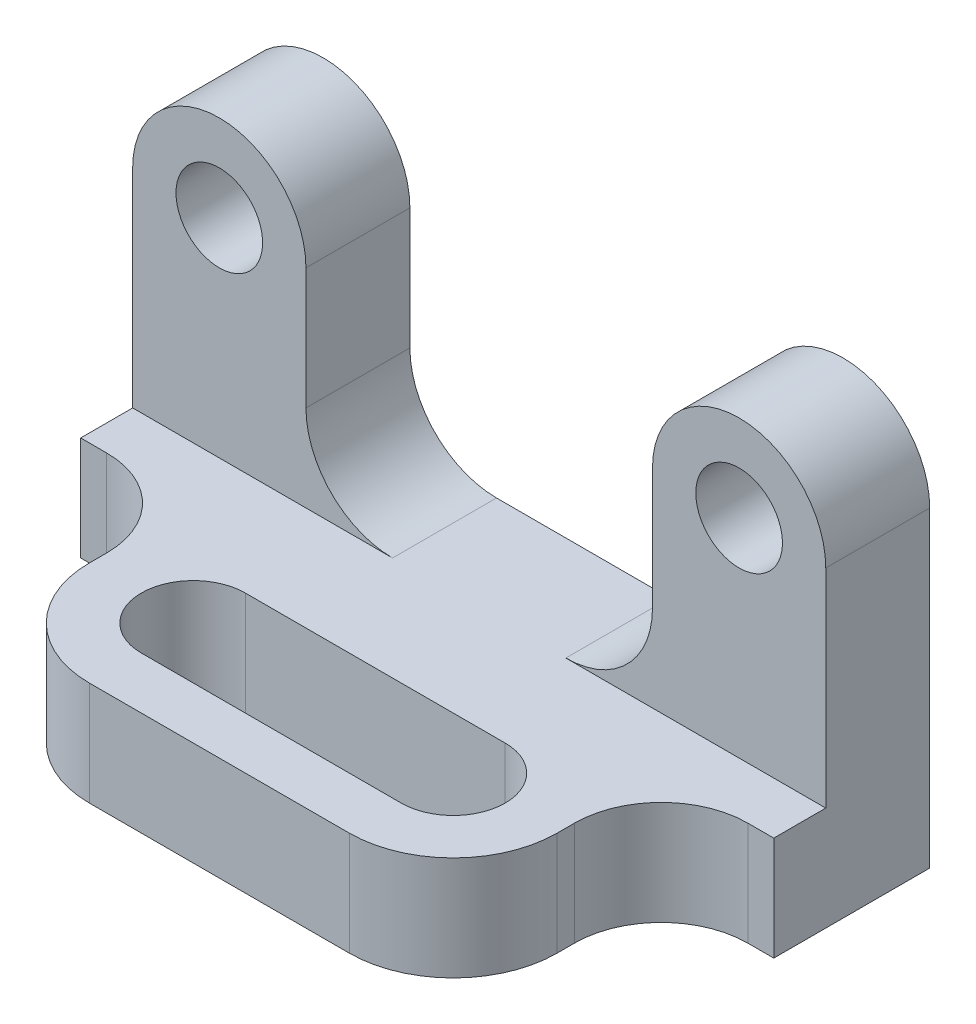
ISO-10303-21;
HEADER;
FILE_DESCRIPTION(('STEP AP214'),'2;1');
FILE_NAME('part.step','',(''),(''),'','','');
FILE_SCHEMA(('AUTOMOTIVE_DESIGN { 1 0 10303 214 1 1 1 1 }'));
ENDSEC;
DATA;
#1=APPLICATION_CONTEXT('core data for automotive mechanical design processes');
#2=APPLICATION_PROTOCOL_DEFINITION('international standard','automotive_design',2000,#1);
#3=PRODUCT_CONTEXT('',#1,'mechanical');
#4=PRODUCT('Part','Part','',(#3));
#5=PRODUCT_RELATED_PRODUCT_CATEGORY('part','',(#4));
#6=PRODUCT_DEFINITION_FORMATION('','',#4);
#7=PRODUCT_DEFINITION_CONTEXT('part definition',#1,'design');
#8=PRODUCT_DEFINITION('design','',#6,#7);
#9=PRODUCT_DEFINITION_SHAPE('','',#8);
#10=(LENGTH_UNIT() NAMED_UNIT(*) SI_UNIT(.MILLI.,.METRE.));
#11=(NAMED_UNIT(*) PLANE_ANGLE_UNIT() SI_UNIT($,.RADIAN.));
#12=(NAMED_UNIT(*) SI_UNIT($,.STERADIAN.) SOLID_ANGLE_UNIT());
#13=UNCERTAINTY_MEASURE_WITH_UNIT(LENGTH_MEASURE(1.E-05),#10,'distance_accuracy_value','');
#14=(GEOMETRIC_REPRESENTATION_CONTEXT(3) GLOBAL_UNCERTAINTY_ASSIGNED_CONTEXT((#13)) GLOBAL_UNIT_ASSIGNED_CONTEXT((#10,
#11,#12)) REPRESENTATION_CONTEXT('',''));
#15=CARTESIAN_POINT('',(0.,0.,0.));
#16=DIRECTION('',(0.,0.,1.));
#17=DIRECTION('',(1.,0.,0.));
#18=AXIS2_PLACEMENT_3D('',#15,#16,#17);
#19=CARTESIAN_POINT('',(0.,3.,0.));
#20=DIRECTION('',(0.,1.,0.));
#21=DIRECTION('',(0.,0.,1.));
#22=AXIS2_PLACEMENT_3D('',#19,#20,#21);
#23=PLANE('',#22);
#24=CARTESIAN_POINT('',(7.5,3.,12.));
#25=DIRECTION('',(0.,1.,0.));
#26=DIRECTION('',(0.,0.,1.));
#27=AXIS2_PLACEMENT_3D('',#24,#25,#26);
#28=CIRCLE('',#27,3.);
#29=CARTESIAN_POINT('',(7.5,3.,15.));
#30=VERTEX_POINT('',#29);
#31=CARTESIAN_POINT('',(7.5,3.,8.99999999999999));
#32=VERTEX_POINT('',#31);
#33=EDGE_CURVE('E176',#30,#32,#28,.T.);
#34=ORIENTED_EDGE('',*,*,#33,.F.);
#35=DIRECTION('',(1.,0.,0.));
#36=VECTOR('',#35,1.);
#37=CARTESIAN_POINT('',(0.,3.,15.));
#38=LINE('',#37,#36);
#39=CARTESIAN_POINT('',(-7.5,3.,15.));
#40=VERTEX_POINT('',#39);
#41=EDGE_CURVE('E164',#40,#30,#38,.T.);
#42=ORIENTED_EDGE('',*,*,#41,.F.);
#43=CARTESIAN_POINT('',(-7.5,3.,12.));
#44=DIRECTION('',(0.,1.,0.));
#45=DIRECTION('',(0.,0.,1.));
#46=AXIS2_PLACEMENT_3D('',#43,#44,#45);
#47=CIRCLE('',#46,3.);
#48=CARTESIAN_POINT('',(-7.5,3.,8.99999999999999));
#49=VERTEX_POINT('',#48);
#50=EDGE_CURVE('E179',#49,#40,#47,.T.);
#51=ORIENTED_EDGE('',*,*,#50,.F.);
#52=DIRECTION('',(1.,0.,0.));
#53=VECTOR('',#52,1.);
#54=CARTESIAN_POINT('',(0.,3.,8.99999999999999));
#55=LINE('',#54,#53);
#56=EDGE_CURVE('E64',#49,#32,#55,.T.);
#57=ORIENTED_EDGE('',*,*,#56,.T.);
#58=EDGE_LOOP('',(#34,#42,#51,#57));
#59=FACE_BOUND('',#58,.T.);
#60=DIRECTION('',(0.,0.,-1.));
#61=VECTOR('',#60,1.);
#62=CARTESIAN_POINT('',(20.,3.,0.));
#63=LINE('',#62,#61);
#64=CARTESIAN_POINT('',(20.,3.,5.99999999999999));
#65=VERTEX_POINT('',#64);
#66=CARTESIAN_POINT('',(20.,3.,3.));
#67=VERTEX_POINT('',#66);
#68=EDGE_CURVE('E354',#65,#67,#63,.T.);
#69=ORIENTED_EDGE('',*,*,#68,.T.);
#70=DIRECTION('',(-1.,0.,0.));
#71=VECTOR('',#70,1.);
#72=CARTESIAN_POINT('',(0.,3.,3.));
#73=LINE('',#72,#71);
#74=CARTESIAN_POINT('',(4.99999999999997,3.,3.));
#75=VERTEX_POINT('',#74);
#76=EDGE_CURVE('E188',#67,#75,#73,.T.);
#77=ORIENTED_EDGE('',*,*,#76,.T.);
#78=DIRECTION('',(0.,0.,1.));
#79=VECTOR('',#78,1.);
#80=CARTESIAN_POINT('',(5.,3.,-3.));
#81=LINE('',#80,#79);
#82=CARTESIAN_POINT('',(4.99999999999997,3.,-3.));
#83=VERTEX_POINT('',#82);
#84=EDGE_CURVE('E47',#75,#83,#81,.F.);
#85=ORIENTED_EDGE('',*,*,#84,.T.);
#86=DIRECTION('',(1.,0.,0.));
#87=VECTOR('',#86,1.);
#88=CARTESIAN_POINT('',(0.,3.,-3.));
#89=LINE('',#88,#87);
#90=CARTESIAN_POINT('',(-4.99999999999997,3.,-3.));
#91=VERTEX_POINT('',#90);
#92=EDGE_CURVE('E260',#91,#83,#89,.T.);
#93=ORIENTED_EDGE('',*,*,#92,.F.);
#94=DIRECTION('',(0.,0.,1.));
#95=VECTOR('',#94,1.);
#96=CARTESIAN_POINT('',(-5.,3.,-3.));
#97=LINE('',#96,#95);
#98=CARTESIAN_POINT('',(-4.99999999999997,3.,3.));
#99=VERTEX_POINT('',#98);
#100=EDGE_CURVE('E11',#99,#91,#97,.F.);
#101=ORIENTED_EDGE('',*,*,#100,.F.);
#102=CARTESIAN_POINT('',(-20.,3.,3.));
#103=VERTEX_POINT('',#102);
#104=EDGE_CURVE('E344',#99,#103,#73,.T.);
#105=ORIENTED_EDGE('',*,*,#104,.T.);
#106=DIRECTION('',(0.,0.,1.));
#107=VECTOR('',#106,1.);
#108=CARTESIAN_POINT('',(-20.,3.,0.));
#109=LINE('',#108,#107);
#110=CARTESIAN_POINT('',(-20.,3.,6.));
#111=VERTEX_POINT('',#110);
#112=EDGE_CURVE('E356',#103,#111,#109,.T.);
#113=ORIENTED_EDGE('',*,*,#112,.T.);
#114=DIRECTION('',(1.,0.,0.));
#115=VECTOR('',#114,1.);
#116=CARTESIAN_POINT('',(0.,3.,6.));
#117=LINE('',#116,#115);
#118=CARTESIAN_POINT('',(-18.5,3.,6.));
#119=VERTEX_POINT('',#118);
#120=EDGE_CURVE('E358',#111,#119,#117,.T.);
#121=ORIENTED_EDGE('',*,*,#120,.T.);
#122=CARTESIAN_POINT('',(-18.5,3.,11.));
#123=DIRECTION('',(0.,1.,0.));
#124=DIRECTION('',(0.,0.,1.));
#125=AXIS2_PLACEMENT_3D('',#122,#123,#124);
#126=CIRCLE('',#125,5.);
#127=CARTESIAN_POINT('',(-13.5,3.,11.));
#128=VERTEX_POINT('',#127);
#129=EDGE_CURVE('E363',#128,#119,#126,.T.);
#130=ORIENTED_EDGE('',*,*,#129,.F.);
#131=DIRECTION('',(0.,0.,-1.));
#132=VECTOR('',#131,1.);
#133=CARTESIAN_POINT('',(-13.5,3.,0.));
#134=LINE('',#133,#132);
#135=CARTESIAN_POINT('',(-13.5,3.,12.));
#136=VERTEX_POINT('',#135);
#137=EDGE_CURVE('E365',#136,#128,#134,.T.);
#138=ORIENTED_EDGE('',*,*,#137,.F.);
#139=CARTESIAN_POINT('',(-7.5,3.,12.));
#140=DIRECTION('',(0.,1.,0.));
#141=DIRECTION('',(0.,0.,1.));
#142=AXIS2_PLACEMENT_3D('',#139,#140,#141);
#143=CIRCLE('',#142,6.);
#144=CARTESIAN_POINT('',(-7.49999999999996,3.,18.));
#145=VERTEX_POINT('',#144);
#146=EDGE_CURVE('E224',#145,#136,#143,.F.);
#147=ORIENTED_EDGE('',*,*,#146,.F.);
#148=DIRECTION('',(1.,0.,0.));
#149=VECTOR('',#148,1.);
#150=CARTESIAN_POINT('',(0.,3.,18.));
#151=LINE('',#150,#149);
#152=CARTESIAN_POINT('',(7.49999999999996,3.,18.));
#153=VERTEX_POINT('',#152);
#154=EDGE_CURVE('E343',#145,#153,#151,.T.);
#155=ORIENTED_EDGE('',*,*,#154,.T.);
#156=CARTESIAN_POINT('',(7.5,3.,12.));
#157=DIRECTION('',(0.,1.,0.));
#158=DIRECTION('',(0.,0.,1.));
#159=AXIS2_PLACEMENT_3D('',#156,#157,#158);
#160=CIRCLE('',#159,6.);
#161=CARTESIAN_POINT('',(13.5,3.,12.));
#162=VERTEX_POINT('',#161);
#163=EDGE_CURVE('E347',#162,#153,#160,.F.);
#164=ORIENTED_EDGE('',*,*,#163,.F.);
#165=DIRECTION('',(0.,0.,-1.));
#166=VECTOR('',#165,1.);
#167=CARTESIAN_POINT('',(13.5,3.,0.));
#168=LINE('',#167,#166);
#169=CARTESIAN_POINT('',(13.5,3.,11.));
#170=VERTEX_POINT('',#169);
#171=EDGE_CURVE('E349',#162,#170,#168,.T.);
#172=ORIENTED_EDGE('',*,*,#171,.T.);
#173=CARTESIAN_POINT('',(18.5,3.,11.));
#174=DIRECTION('',(0.,1.,0.));
#175=DIRECTION('',(0.,0.,1.));
#176=AXIS2_PLACEMENT_3D('',#173,#174,#175);
#177=CIRCLE('',#176,5.);
#178=CARTESIAN_POINT('',(18.5,3.,5.99999999999999));
#179=VERTEX_POINT('',#178);
#180=EDGE_CURVE('E351',#170,#179,#177,.F.);
#181=ORIENTED_EDGE('',*,*,#180,.T.);
#182=DIRECTION('',(1.,0.,0.));
#183=VECTOR('',#182,1.);
#184=CARTESIAN_POINT('',(0.,3.,5.99999999999999));
#185=LINE('',#184,#183);
#186=EDGE_CURVE('E352',#179,#65,#185,.T.);
#187=ORIENTED_EDGE('',*,*,#186,.T.);
#188=EDGE_LOOP('',(#69,#77,#85,#93,#101,#105,#113,#121,#130,#138,#147,#155,#164,#172,#181,#187));
#189=FACE_BOUND('',#188,.T.);
#190=ADVANCED_FACE('F41',(#59,#189),#23,.T.);
#191=CARTESIAN_POINT('',(7.5,3.,12.));
#192=DIRECTION('',(0.,-1.,0.));
#193=DIRECTION('',(0.,0.,-1.));
#194=AXIS2_PLACEMENT_3D('',#191,#192,#193);
#195=CYLINDRICAL_SURFACE('',#194,3.);
#196=CARTESIAN_POINT('',(7.5,-3.,12.));
#197=DIRECTION('',(0.,1.,0.));
#198=DIRECTION('',(0.,0.,1.));
#199=AXIS2_PLACEMENT_3D('',#196,#197,#198);
#200=CIRCLE('',#199,3.);
#201=CARTESIAN_POINT('',(7.5,-3.,15.));
#202=VERTEX_POINT('',#201);
#203=CARTESIAN_POINT('',(7.5,-3.,8.99999999999999));
#204=VERTEX_POINT('',#203);
#205=EDGE_CURVE('E214',#202,#204,#200,.T.);
#206=ORIENTED_EDGE('',*,*,#205,.F.);
#207=DIRECTION('',(0.,-1.,0.));
#208=VECTOR('',#207,1.);
#209=CARTESIAN_POINT('',(7.5,3.,15.));
#210=LINE('',#209,#208);
#211=EDGE_CURVE('E175',#30,#202,#210,.T.);
#212=ORIENTED_EDGE('',*,*,#211,.F.);
#213=ORIENTED_EDGE('',*,*,#33,.T.);
#214=DIRECTION('',(0.,-1.,0.));
#215=VECTOR('',#214,1.);
#216=CARTESIAN_POINT('',(7.5,3.,8.99999999999999));
#217=LINE('',#216,#215);
#218=EDGE_CURVE('E120',#32,#204,#217,.T.);
#219=ORIENTED_EDGE('',*,*,#218,.T.);
#220=EDGE_LOOP('',(#206,#212,#213,#219));
#221=FACE_BOUND('',#220,.T.);
#222=ADVANCED_FACE('F368',(#221),#195,.F.);
#223=CARTESIAN_POINT('',(0.,3.,15.));
#224=DIRECTION('',(0.,0.,-1.));
#225=DIRECTION('',(-1.,0.,0.));
#226=AXIS2_PLACEMENT_3D('',#223,#224,#225);
#227=PLANE('',#226);
#228=DIRECTION('',(1.,0.,0.));
#229=VECTOR('',#228,1.);
#230=CARTESIAN_POINT('',(0.,-3.,15.));
#231=LINE('',#230,#229);
#232=CARTESIAN_POINT('',(-7.5,-3.,15.));
#233=VERTEX_POINT('',#232);
#234=EDGE_CURVE('E170',#233,#202,#231,.T.);
#235=ORIENTED_EDGE('',*,*,#234,.F.);
#236=DIRECTION('',(0.,-1.,0.));
#237=VECTOR('',#236,1.);
#238=CARTESIAN_POINT('',(-7.5,3.,15.));
#239=LINE('',#238,#237);
#240=EDGE_CURVE('E165',#40,#233,#239,.T.);
#241=ORIENTED_EDGE('',*,*,#240,.F.);
#242=ORIENTED_EDGE('',*,*,#41,.T.);
#243=ORIENTED_EDGE('',*,*,#211,.T.);
#244=EDGE_LOOP('',(#235,#241,#242,#243));
#245=FACE_BOUND('',#244,.T.);
#246=ADVANCED_FACE('F163',(#245),#227,.T.);
#247=CARTESIAN_POINT('',(-7.5,3.,12.));
#248=DIRECTION('',(0.,-1.,0.));
#249=DIRECTION('',(0.,0.,-1.));
#250=AXIS2_PLACEMENT_3D('',#247,#248,#249);
#251=CYLINDRICAL_SURFACE('',#250,3.);
#252=CARTESIAN_POINT('',(-7.5,-3.,12.));
#253=DIRECTION('',(0.,1.,0.));
#254=DIRECTION('',(0.,0.,1.));
#255=AXIS2_PLACEMENT_3D('',#252,#253,#254);
#256=CIRCLE('',#255,3.);
#257=CARTESIAN_POINT('',(-7.5,-3.,8.99999999999999));
#258=VERTEX_POINT('',#257);
#259=EDGE_CURVE('E218',#258,#233,#256,.T.);
#260=ORIENTED_EDGE('',*,*,#259,.F.);
#261=DIRECTION('',(0.,-1.,0.));
#262=VECTOR('',#261,1.);
#263=CARTESIAN_POINT('',(-7.5,3.,8.99999999999999));
#264=LINE('',#263,#262);
#265=EDGE_CURVE('E172',#49,#258,#264,.T.);
#266=ORIENTED_EDGE('',*,*,#265,.F.);
#267=ORIENTED_EDGE('',*,*,#50,.T.);
#268=ORIENTED_EDGE('',*,*,#240,.T.);
#269=EDGE_LOOP('',(#260,#266,#267,#268));
#270=FACE_BOUND('',#269,.T.);
#271=ADVANCED_FACE('F178',(#270),#251,.F.);
#272=CARTESIAN_POINT('',(-7.5,3.,12.));
#273=DIRECTION('',(0.,-1.,0.));
#274=DIRECTION('',(0.,0.,-1.));
#275=AXIS2_PLACEMENT_3D('',#272,#273,#274);
#276=CYLINDRICAL_SURFACE('',#275,6.);
#277=CARTESIAN_POINT('',(-7.5,-3.,12.));
#278=DIRECTION('',(0.,1.,0.));
#279=DIRECTION('',(0.,0.,1.));
#280=AXIS2_PLACEMENT_3D('',#277,#278,#279);
#281=CIRCLE('',#280,6.);
#282=CARTESIAN_POINT('',(-7.49999999999996,-3.,18.));
#283=VERTEX_POINT('',#282);
#284=CARTESIAN_POINT('',(-13.5,-3.,12.));
#285=VERTEX_POINT('',#284);
#286=EDGE_CURVE('E183',#283,#285,#281,.F.);
#287=ORIENTED_EDGE('',*,*,#286,.F.);
#288=DIRECTION('',(0.,-1.,0.));
#289=VECTOR('',#288,1.);
#290=CARTESIAN_POINT('',(-7.49999999999996,3.,18.));
#291=LINE('',#290,#289);
#292=EDGE_CURVE('E122',#145,#283,#291,.T.);
#293=ORIENTED_EDGE('',*,*,#292,.F.);
#294=ORIENTED_EDGE('',*,*,#146,.T.);
#295=DIRECTION('',(0.,-1.,0.));
#296=VECTOR('',#295,1.);
#297=CARTESIAN_POINT('',(-13.5,3.,12.));
#298=LINE('',#297,#296);
#299=EDGE_CURVE('E182',#136,#285,#298,.T.);
#300=ORIENTED_EDGE('',*,*,#299,.T.);
#301=EDGE_LOOP('',(#287,#293,#294,#300));
#302=FACE_BOUND('',#301,.T.);
#303=ADVANCED_FACE('F43',(#302),#276,.T.);
#304=CARTESIAN_POINT('',(0.,3.,18.));
#305=DIRECTION('',(0.,0.,-1.));
#306=DIRECTION('',(-1.,0.,0.));
#307=AXIS2_PLACEMENT_3D('',#304,#305,#306);
#308=PLANE('',#307);
#309=DIRECTION('',(1.,0.,0.));
#310=VECTOR('',#309,1.);
#311=CARTESIAN_POINT('',(0.,-3.,18.));
#312=LINE('',#311,#310);
#313=CARTESIAN_POINT('',(7.49999999999996,-3.,18.));
#314=VERTEX_POINT('',#313);
#315=EDGE_CURVE('E187',#283,#314,#312,.T.);
#316=ORIENTED_EDGE('',*,*,#315,.T.);
#317=DIRECTION('',(0.,-1.,0.));
#318=VECTOR('',#317,1.);
#319=CARTESIAN_POINT('',(7.49999999999996,3.,18.));
#320=LINE('',#319,#318);
#321=EDGE_CURVE('E249',#153,#314,#320,.T.);
#322=ORIENTED_EDGE('',*,*,#321,.F.);
#323=ORIENTED_EDGE('',*,*,#154,.F.);
#324=ORIENTED_EDGE('',*,*,#292,.T.);
#325=EDGE_LOOP('',(#316,#322,#323,#324));
#326=FACE_BOUND('',#325,.T.);
#327=ADVANCED_FACE('F601',(#326),#308,.F.);
#328=CARTESIAN_POINT('',(7.5,3.,12.));
#329=DIRECTION('',(0.,-1.,0.));
#330=DIRECTION('',(0.,0.,-1.));
#331=AXIS2_PLACEMENT_3D('',#328,#329,#330);
#332=CYLINDRICAL_SURFACE('',#331,6.);
#333=CARTESIAN_POINT('',(7.5,-3.,12.));
#334=DIRECTION('',(0.,1.,0.));
#335=DIRECTION('',(0.,0.,1.));
#336=AXIS2_PLACEMENT_3D('',#333,#334,#335);
#337=CIRCLE('',#336,6.);
#338=CARTESIAN_POINT('',(13.5,-3.,12.));
#339=VERTEX_POINT('',#338);
#340=EDGE_CURVE('E191',#339,#314,#337,.F.);
#341=ORIENTED_EDGE('',*,*,#340,.F.);
#342=DIRECTION('',(0.,-1.,0.));
#343=VECTOR('',#342,1.);
#344=CARTESIAN_POINT('',(13.5,3.,12.));
#345=LINE('',#344,#343);
#346=EDGE_CURVE('E243',#162,#339,#345,.T.);
#347=ORIENTED_EDGE('',*,*,#346,.F.);
#348=ORIENTED_EDGE('',*,*,#163,.T.);
#349=ORIENTED_EDGE('',*,*,#321,.T.);
#350=EDGE_LOOP('',(#341,#347,#348,#349));
#351=FACE_BOUND('',#350,.T.);
#352=ADVANCED_FACE('F595',(#351),#332,.T.);
#353=CARTESIAN_POINT('',(13.5,3.,0.));
#354=DIRECTION('',(-1.,0.,0.));
#355=DIRECTION('',(0.,0.,1.));
#356=AXIS2_PLACEMENT_3D('',#353,#354,#355);
#357=PLANE('',#356);
#358=DIRECTION('',(0.,0.,-1.));
#359=VECTOR('',#358,1.);
#360=CARTESIAN_POINT('',(13.5,-3.,0.));
#361=LINE('',#360,#359);
#362=CARTESIAN_POINT('',(13.5,-3.,11.));
#363=VERTEX_POINT('',#362);
#364=EDGE_CURVE('E192',#339,#363,#361,.T.);
#365=ORIENTED_EDGE('',*,*,#364,.T.);
#366=DIRECTION('',(0.,-1.,0.));
#367=VECTOR('',#366,1.);
#368=CARTESIAN_POINT('',(13.5,3.,11.));
#369=LINE('',#368,#367);
#370=EDGE_CURVE('E241',#170,#363,#369,.T.);
#371=ORIENTED_EDGE('',*,*,#370,.F.);
#372=ORIENTED_EDGE('',*,*,#171,.F.);
#373=ORIENTED_EDGE('',*,*,#346,.T.);
#374=EDGE_LOOP('',(#365,#371,#372,#373));
#375=FACE_BOUND('',#374,.T.);
#376=ADVANCED_FACE('F581',(#375),#357,.F.);
#377=CARTESIAN_POINT('',(18.5,3.,11.));
#378=DIRECTION('',(0.,-1.,0.));
#379=DIRECTION('',(0.,0.,-1.));
#380=AXIS2_PLACEMENT_3D('',#377,#378,#379);
#381=CYLINDRICAL_SURFACE('',#380,5.);
#382=CARTESIAN_POINT('',(18.5,-3.,11.));
#383=DIRECTION('',(0.,1.,0.));
#384=DIRECTION('',(0.,0.,1.));
#385=AXIS2_PLACEMENT_3D('',#382,#383,#384);
#386=CIRCLE('',#385,5.);
#387=CARTESIAN_POINT('',(18.5,-3.,5.99999999999999));
#388=VERTEX_POINT('',#387);
#389=EDGE_CURVE('E197',#363,#388,#386,.F.);
#390=ORIENTED_EDGE('',*,*,#389,.T.);
#391=DIRECTION('',(0.,-1.,0.));
#392=VECTOR('',#391,1.);
#393=CARTESIAN_POINT('',(18.5,3.,5.99999999999999));
#394=LINE('',#393,#392);
#395=EDGE_CURVE('E236',#179,#388,#394,.T.);
#396=ORIENTED_EDGE('',*,*,#395,.F.);
#397=ORIENTED_EDGE('',*,*,#180,.F.);
#398=ORIENTED_EDGE('',*,*,#370,.T.);
#399=EDGE_LOOP('',(#390,#396,#397,#398));
#400=FACE_BOUND('',#399,.T.);
#401=ADVANCED_FACE('F573',(#400),#381,.F.);
#402=CARTESIAN_POINT('',(0.,3.,5.99999999999999));
#403=DIRECTION('',(0.,0.,-1.));
#404=DIRECTION('',(-1.,0.,0.));
#405=AXIS2_PLACEMENT_3D('',#402,#403,#404);
#406=PLANE('',#405);
#407=DIRECTION('',(1.,0.,0.));
#408=VECTOR('',#407,1.);
#409=CARTESIAN_POINT('',(0.,-3.,5.99999999999999));
#410=LINE('',#409,#408);
#411=CARTESIAN_POINT('',(20.,-3.,5.99999999999999));
#412=VERTEX_POINT('',#411);
#413=EDGE_CURVE('E200',#388,#412,#410,.T.);
#414=ORIENTED_EDGE('',*,*,#413,.T.);
#415=DIRECTION('',(0.,-1.,0.));
#416=VECTOR('',#415,1.);
#417=CARTESIAN_POINT('',(20.,3.,5.99999999999999));
#418=LINE('',#417,#416);
#419=EDGE_CURVE('E232',#65,#412,#418,.T.);
#420=ORIENTED_EDGE('',*,*,#419,.F.);
#421=ORIENTED_EDGE('',*,*,#186,.F.);
#422=ORIENTED_EDGE('',*,*,#395,.T.);
#423=EDGE_LOOP('',(#414,#420,#421,#422));
#424=FACE_BOUND('',#423,.T.);
#425=ADVANCED_FACE('F563',(#424),#406,.F.);
#426=CARTESIAN_POINT('',(20.,3.,0.));
#427=DIRECTION('',(-1.,0.,0.));
#428=DIRECTION('',(0.,0.,1.));
#429=AXIS2_PLACEMENT_3D('',#426,#427,#428);
#430=PLANE('',#429);
#431=DIRECTION('',(0.,0.,-1.));
#432=VECTOR('',#431,1.);
#433=CARTESIAN_POINT('',(20.,-3.,0.));
#434=LINE('',#433,#432);
#435=CARTESIAN_POINT('',(20.,-3.,-3.));
#436=VERTEX_POINT('',#435);
#437=EDGE_CURVE('E203',#412,#436,#434,.T.);
#438=ORIENTED_EDGE('',*,*,#437,.T.);
#439=DIRECTION('',(0.,-1.,0.));
#440=VECTOR('',#439,1.);
#441=CARTESIAN_POINT('',(20.,0.,-3.));
#442=LINE('',#441,#440);
#443=CARTESIAN_POINT('',(20.,15.,-3.));
#444=VERTEX_POINT('',#443);
#445=EDGE_CURVE('E324',#444,#436,#442,.T.);
#446=ORIENTED_EDGE('',*,*,#445,.F.);
#447=DIRECTION('',(0.,0.,1.));
#448=VECTOR('',#447,1.);
#449=CARTESIAN_POINT('',(20.,15.,-3.));
#450=LINE('',#449,#448);
#451=CARTESIAN_POINT('',(20.,15.,3.));
#452=VERTEX_POINT('',#451);
#453=EDGE_CURVE('E300',#444,#452,#450,.T.);
#454=ORIENTED_EDGE('',*,*,#453,.T.);
#455=DIRECTION('',(0.,-1.,0.));
#456=VECTOR('',#455,1.);
#457=CARTESIAN_POINT('',(20.,0.,3.));
#458=LINE('',#457,#456);
#459=EDGE_CURVE('E297',#452,#67,#458,.T.);
#460=ORIENTED_EDGE('',*,*,#459,.T.);
#461=ORIENTED_EDGE('',*,*,#68,.F.);
#462=ORIENTED_EDGE('',*,*,#419,.T.);
#463=EDGE_LOOP('',(#438,#446,#454,#460,#461,#462));
#464=FACE_BOUND('',#463,.T.);
#465=ADVANCED_FACE('F553',(#464),#430,.F.);
#466=CARTESIAN_POINT('',(-20.,3.,0.));
#467=DIRECTION('',(1.,0.,0.));
#468=DIRECTION('',(0.,0.,-1.));
#469=AXIS2_PLACEMENT_3D('',#466,#467,#468);
#470=PLANE('',#469);
#471=DIRECTION('',(0.,1.,0.));
#472=VECTOR('',#471,1.);
#473=CARTESIAN_POINT('',(-20.,0.,-3.));
#474=LINE('',#473,#472);
#475=CARTESIAN_POINT('',(-20.,-3.,-3.));
#476=VERTEX_POINT('',#475);
#477=CARTESIAN_POINT('',(-20.,15.,-3.));
#478=VERTEX_POINT('',#477);
#479=EDGE_CURVE('E663',#476,#478,#474,.T.);
#480=ORIENTED_EDGE('',*,*,#479,.F.);
#481=DIRECTION('',(0.,0.,1.));
#482=VECTOR('',#481,1.);
#483=CARTESIAN_POINT('',(-20.,-3.,0.));
#484=LINE('',#483,#482);
#485=CARTESIAN_POINT('',(-20.,-3.,6.));
#486=VERTEX_POINT('',#485);
#487=EDGE_CURVE('E204',#476,#486,#484,.T.);
#488=ORIENTED_EDGE('',*,*,#487,.T.);
#489=DIRECTION('',(0.,-1.,0.));
#490=VECTOR('',#489,1.);
#491=CARTESIAN_POINT('',(-20.,3.,6.));
#492=LINE('',#491,#490);
#493=EDGE_CURVE('E231',#111,#486,#492,.T.);
#494=ORIENTED_EDGE('',*,*,#493,.F.);
#495=ORIENTED_EDGE('',*,*,#112,.F.);
#496=DIRECTION('',(0.,1.,0.));
#497=VECTOR('',#496,1.);
#498=CARTESIAN_POINT('',(-20.,0.,3.));
#499=LINE('',#498,#497);
#500=CARTESIAN_POINT('',(-20.,15.,3.));
#501=VERTEX_POINT('',#500);
#502=EDGE_CURVE('E57',#103,#501,#499,.T.);
#503=ORIENTED_EDGE('',*,*,#502,.T.);
#504=DIRECTION('',(0.,0.,1.));
#505=VECTOR('',#504,1.);
#506=CARTESIAN_POINT('',(-20.,15.,-3.));
#507=LINE('',#506,#505);
#508=EDGE_CURVE('E337',#478,#501,#507,.T.);
#509=ORIENTED_EDGE('',*,*,#508,.F.);
#510=EDGE_LOOP('',(#480,#488,#494,#495,#503,#509));
#511=FACE_BOUND('',#510,.T.);
#512=ADVANCED_FACE('F546',(#511),#470,.F.);
#513=CARTESIAN_POINT('',(0.,3.,6.));
#514=DIRECTION('',(0.,0.,-1.));
#515=DIRECTION('',(-1.,0.,0.));
#516=AXIS2_PLACEMENT_3D('',#513,#514,#515);
#517=PLANE('',#516);
#518=DIRECTION('',(1.,0.,0.));
#519=VECTOR('',#518,1.);
#520=CARTESIAN_POINT('',(0.,-3.,6.));
#521=LINE('',#520,#519);
#522=CARTESIAN_POINT('',(-18.5,-3.,6.));
#523=VERTEX_POINT('',#522);
#524=EDGE_CURVE('E206',#486,#523,#521,.T.);
#525=ORIENTED_EDGE('',*,*,#524,.T.);
#526=DIRECTION('',(0.,-1.,0.));
#527=VECTOR('',#526,1.);
#528=CARTESIAN_POINT('',(-18.5,3.,6.));
#529=LINE('',#528,#527);
#530=EDGE_CURVE('E229',#119,#523,#529,.T.);
#531=ORIENTED_EDGE('',*,*,#530,.F.);
#532=ORIENTED_EDGE('',*,*,#120,.F.);
#533=ORIENTED_EDGE('',*,*,#493,.T.);
#534=EDGE_LOOP('',(#525,#531,#532,#533));
#535=FACE_BOUND('',#534,.T.);
#536=ADVANCED_FACE('F540',(#535),#517,.F.);
#537=CARTESIAN_POINT('',(-18.5,3.,11.));
#538=DIRECTION('',(0.,-1.,0.));
#539=DIRECTION('',(0.,0.,-1.));
#540=AXIS2_PLACEMENT_3D('',#537,#538,#539);
#541=CYLINDRICAL_SURFACE('',#540,5.);
#542=CARTESIAN_POINT('',(-18.5,-3.,11.));
#543=DIRECTION('',(0.,1.,0.));
#544=DIRECTION('',(0.,0.,1.));
#545=AXIS2_PLACEMENT_3D('',#542,#543,#544);
#546=CIRCLE('',#545,5.);
#547=CARTESIAN_POINT('',(-13.5,-3.,11.));
#548=VERTEX_POINT('',#547);
#549=EDGE_CURVE('E207',#548,#523,#546,.T.);
#550=ORIENTED_EDGE('',*,*,#549,.F.);
#551=DIRECTION('',(0.,-1.,0.));
#552=VECTOR('',#551,1.);
#553=CARTESIAN_POINT('',(-13.5,3.,11.));
#554=LINE('',#553,#552);
#555=EDGE_CURVE('E227',#128,#548,#554,.T.);
#556=ORIENTED_EDGE('',*,*,#555,.F.);
#557=ORIENTED_EDGE('',*,*,#129,.T.);
#558=ORIENTED_EDGE('',*,*,#530,.T.);
#559=EDGE_LOOP('',(#550,#556,#557,#558));
#560=FACE_BOUND('',#559,.T.);
#561=ADVANCED_FACE('F382',(#560),#541,.F.);
#562=CARTESIAN_POINT('',(-13.5,3.,0.));
#563=DIRECTION('',(-1.,0.,0.));
#564=DIRECTION('',(0.,0.,1.));
#565=AXIS2_PLACEMENT_3D('',#562,#563,#564);
#566=PLANE('',#565);
#567=DIRECTION('',(0.,0.,-1.));
#568=VECTOR('',#567,1.);
#569=CARTESIAN_POINT('',(-13.5,-3.,0.));
#570=LINE('',#569,#568);
#571=EDGE_CURVE('E215',#285,#548,#570,.T.);
#572=ORIENTED_EDGE('',*,*,#571,.F.);
#573=ORIENTED_EDGE('',*,*,#299,.F.);
#574=ORIENTED_EDGE('',*,*,#137,.T.);
#575=ORIENTED_EDGE('',*,*,#555,.T.);
#576=EDGE_LOOP('',(#572,#573,#574,#575));
#577=FACE_BOUND('',#576,.T.);
#578=ADVANCED_FACE('F373',(#577),#566,.T.);
#579=CARTESIAN_POINT('',(0.,3.,8.99999999999999));
#580=DIRECTION('',(0.,0.,-1.));
#581=DIRECTION('',(-1.,0.,0.));
#582=AXIS2_PLACEMENT_3D('',#579,#580,#581);
#583=PLANE('',#582);
#584=DIRECTION('',(1.,0.,0.));
#585=VECTOR('',#584,1.);
#586=CARTESIAN_POINT('',(0.,-3.,8.99999999999999));
#587=LINE('',#586,#585);
#588=EDGE_CURVE('E222',#258,#204,#587,.T.);
#589=ORIENTED_EDGE('',*,*,#588,.T.);
#590=ORIENTED_EDGE('',*,*,#218,.F.);
#591=ORIENTED_EDGE('',*,*,#56,.F.);
#592=ORIENTED_EDGE('',*,*,#265,.T.);
#593=EDGE_LOOP('',(#589,#590,#591,#592));
#594=FACE_BOUND('',#593,.T.);
#595=ADVANCED_FACE('F371',(#594),#583,.F.);
#596=CARTESIAN_POINT('',(0.,-3.,0.));
#597=DIRECTION('',(0.,1.,0.));
#598=DIRECTION('',(0.,0.,1.));
#599=AXIS2_PLACEMENT_3D('',#596,#597,#598);
#600=PLANE('',#599);
#601=DIRECTION('',(-1.,0.,0.));
#602=VECTOR('',#601,1.);
#603=CARTESIAN_POINT('',(0.,-3.,-3.));
#604=LINE('',#603,#602);
#605=EDGE_CURVE('E671',#436,#476,#604,.T.);
#606=ORIENTED_EDGE('',*,*,#605,.F.);
#607=ORIENTED_EDGE('',*,*,#437,.F.);
#608=ORIENTED_EDGE('',*,*,#413,.F.);
#609=ORIENTED_EDGE('',*,*,#389,.F.);
#610=ORIENTED_EDGE('',*,*,#364,.F.);
#611=ORIENTED_EDGE('',*,*,#340,.T.);
#612=ORIENTED_EDGE('',*,*,#315,.F.);
#613=ORIENTED_EDGE('',*,*,#286,.T.);
#614=ORIENTED_EDGE('',*,*,#571,.T.);
#615=ORIENTED_EDGE('',*,*,#549,.T.);
#616=ORIENTED_EDGE('',*,*,#524,.F.);
#617=ORIENTED_EDGE('',*,*,#487,.F.);
#618=EDGE_LOOP('',(#606,#607,#608,#609,#610,#611,#612,#613,#614,#615,#616,#617));
#619=FACE_BOUND('',#618,.T.);
#620=ORIENTED_EDGE('',*,*,#205,.T.);
#621=ORIENTED_EDGE('',*,*,#588,.F.);
#622=ORIENTED_EDGE('',*,*,#259,.T.);
#623=ORIENTED_EDGE('',*,*,#234,.T.);
#624=EDGE_LOOP('',(#620,#621,#622,#623));
#625=FACE_BOUND('',#624,.T.);
#626=ADVANCED_FACE('F369',(#619,#625),#600,.F.);
#627=CARTESIAN_POINT('',(0.,0.,3.));
#628=DIRECTION('',(0.,0.,-1.));
#629=DIRECTION('',(-1.,0.,0.));
#630=AXIS2_PLACEMENT_3D('',#627,#628,#629);
#631=PLANE('',#630);
#632=ORIENTED_EDGE('',*,*,#76,.F.);
#633=ORIENTED_EDGE('',*,*,#459,.F.);
#634=CARTESIAN_POINT('',(15.,15.,3.));
#635=DIRECTION('',(0.,0.,-1.));
#636=DIRECTION('',(-1.,0.,0.));
#637=AXIS2_PLACEMENT_3D('',#634,#635,#636);
#638=CIRCLE('',#637,5.);
#639=CARTESIAN_POINT('',(10.,15.,3.));
#640=VERTEX_POINT('',#639);
#641=EDGE_CURVE('E316',#640,#452,#638,.T.);
#642=ORIENTED_EDGE('',*,*,#641,.F.);
#643=DIRECTION('',(0.,-1.,0.));
#644=VECTOR('',#643,1.);
#645=CARTESIAN_POINT('',(10.,0.,3.));
#646=LINE('',#645,#644);
#647=CARTESIAN_POINT('',(10.,8.00000000000004,3.));
#648=VERTEX_POINT('',#647);
#649=EDGE_CURVE('E311',#640,#648,#646,.T.);
#650=ORIENTED_EDGE('',*,*,#649,.T.);
#651=CARTESIAN_POINT('',(5.,8.,3.));
#652=DIRECTION('',(0.,0.,-1.));
#653=DIRECTION('',(-1.,0.,0.));
#654=AXIS2_PLACEMENT_3D('',#651,#652,#653);
#655=CIRCLE('',#654,5.);
#656=EDGE_CURVE('E313',#648,#75,#655,.T.);
#657=ORIENTED_EDGE('',*,*,#656,.T.);
#658=EDGE_LOOP('',(#632,#633,#642,#650,#657));
#659=FACE_BOUND('',#658,.T.);
#660=CARTESIAN_POINT('',(15.,15.,3.));
#661=DIRECTION('',(0.,0.,-1.));
#662=DIRECTION('',(-1.,0.,0.));
#663=AXIS2_PLACEMENT_3D('',#660,#661,#662);
#664=CIRCLE('',#663,2.5);
#665=CARTESIAN_POINT('',(12.5,15.,3.));
#666=VERTEX_POINT('',#665);
#667=EDGE_CURVE('E325',#666,#666,#664,.T.);
#668=ORIENTED_EDGE('',*,*,#667,.T.);
#669=EDGE_LOOP('',(#668));
#670=FACE_BOUND('',#669,.T.);
#671=ADVANCED_FACE('F379',(#659,#670),#631,.F.);
#672=CARTESIAN_POINT('',(-15.,15.,-3.));
#673=DIRECTION('',(0.,0.,1.));
#674=DIRECTION('',(1.,0.,0.));
#675=AXIS2_PLACEMENT_3D('',#672,#673,#674);
#676=CYLINDRICAL_SURFACE('',#675,5.);
#677=CARTESIAN_POINT('',(-15.,15.,3.));
#678=DIRECTION('',(0.,0.,-1.));
#679=DIRECTION('',(-1.,0.,0.));
#680=AXIS2_PLACEMENT_3D('',#677,#678,#679);
#681=CIRCLE('',#680,5.);
#682=CARTESIAN_POINT('',(-10.,15.,3.));
#683=VERTEX_POINT('',#682);
#684=EDGE_CURVE('E301',#501,#683,#681,.T.);
#685=ORIENTED_EDGE('',*,*,#684,.T.);
#686=DIRECTION('',(0.,0.,1.));
#687=VECTOR('',#686,1.);
#688=CARTESIAN_POINT('',(-10.,15.,-3.));
#689=LINE('',#688,#687);
#690=CARTESIAN_POINT('',(-10.,15.,-3.));
#691=VERTEX_POINT('',#690);
#692=EDGE_CURVE('E333',#691,#683,#689,.T.);
#693=ORIENTED_EDGE('',*,*,#692,.F.);
#694=CARTESIAN_POINT('',(-15.,15.,-3.));
#695=DIRECTION('',(0.,0.,-1.));
#696=DIRECTION('',(-1.,0.,0.));
#697=AXIS2_PLACEMENT_3D('',#694,#695,#696);
#698=CIRCLE('',#697,5.);
#699=EDGE_CURVE('E674',#478,#691,#698,.T.);
#700=ORIENTED_EDGE('',*,*,#699,.F.);
#701=ORIENTED_EDGE('',*,*,#508,.T.);
#702=EDGE_LOOP('',(#685,#693,#700,#701));
#703=FACE_BOUND('',#702,.T.);
#704=ADVANCED_FACE('F393',(#703),#676,.T.);
#705=CARTESIAN_POINT('',(-10.,0.,-3.));
#706=DIRECTION('',(-1.,0.,0.));
#707=DIRECTION('',(0.,0.,1.));
#708=AXIS2_PLACEMENT_3D('',#705,#706,#707);
#709=PLANE('',#708);
#710=DIRECTION('',(0.,-1.,0.));
#711=VECTOR('',#710,1.);
#712=CARTESIAN_POINT('',(-10.,0.,3.));
#713=LINE('',#712,#711);
#714=CARTESIAN_POINT('',(-10.,8.00000000000004,3.));
#715=VERTEX_POINT('',#714);
#716=EDGE_CURVE('E302',#683,#715,#713,.T.);
#717=ORIENTED_EDGE('',*,*,#716,.T.);
#718=DIRECTION('',(0.,0.,1.));
#719=VECTOR('',#718,1.);
#720=CARTESIAN_POINT('',(-10.,8.00000000000004,-3.));
#721=LINE('',#720,#719);
#722=CARTESIAN_POINT('',(-10.,8.00000000000004,-3.));
#723=VERTEX_POINT('',#722);
#724=EDGE_CURVE('E335',#723,#715,#721,.T.);
#725=ORIENTED_EDGE('',*,*,#724,.F.);
#726=DIRECTION('',(0.,-1.,0.));
#727=VECTOR('',#726,1.);
#728=CARTESIAN_POINT('',(-10.,0.,-3.));
#729=LINE('',#728,#727);
#730=EDGE_CURVE('E673',#691,#723,#729,.T.);
#731=ORIENTED_EDGE('',*,*,#730,.F.);
#732=ORIENTED_EDGE('',*,*,#692,.T.);
#733=EDGE_LOOP('',(#717,#725,#731,#732));
#734=FACE_BOUND('',#733,.T.);
#735=ADVANCED_FACE('F396',(#734),#709,.F.);
#736=CARTESIAN_POINT('',(-5.,8.,-3.));
#737=DIRECTION('',(0.,0.,1.));
#738=DIRECTION('',(1.,0.,0.));
#739=AXIS2_PLACEMENT_3D('',#736,#737,#738);
#740=CYLINDRICAL_SURFACE('',#739,5.);
#741=CARTESIAN_POINT('',(-5.,8.,3.));
#742=DIRECTION('',(0.,0.,-1.));
#743=DIRECTION('',(-1.,0.,0.));
#744=AXIS2_PLACEMENT_3D('',#741,#742,#743);
#745=CIRCLE('',#744,5.);
#746=EDGE_CURVE('E306',#99,#715,#745,.T.);
#747=ORIENTED_EDGE('',*,*,#746,.F.);
#748=ORIENTED_EDGE('',*,*,#100,.T.);
#749=CARTESIAN_POINT('',(-5.,8.,-3.));
#750=DIRECTION('',(0.,0.,-1.));
#751=DIRECTION('',(-1.,0.,0.));
#752=AXIS2_PLACEMENT_3D('',#749,#750,#751);
#753=CIRCLE('',#752,5.);
#754=EDGE_CURVE('E280',#91,#723,#753,.T.);
#755=ORIENTED_EDGE('',*,*,#754,.T.);
#756=ORIENTED_EDGE('',*,*,#724,.T.);
#757=EDGE_LOOP('',(#747,#748,#755,#756));
#758=FACE_BOUND('',#757,.T.);
#759=ADVANCED_FACE('F402',(#758),#740,.F.);
#760=CARTESIAN_POINT('',(5.,8.,-3.));
#761=DIRECTION('',(0.,0.,1.));
#762=DIRECTION('',(1.,0.,0.));
#763=AXIS2_PLACEMENT_3D('',#760,#761,#762);
#764=CYLINDRICAL_SURFACE('',#763,5.);
#765=ORIENTED_EDGE('',*,*,#656,.F.);
#766=DIRECTION('',(0.,0.,1.));
#767=VECTOR('',#766,1.);
#768=CARTESIAN_POINT('',(10.,8.00000000000004,-3.));
#769=LINE('',#768,#767);
#770=CARTESIAN_POINT('',(10.,8.00000000000004,-3.));
#771=VERTEX_POINT('',#770);
#772=EDGE_CURVE('E285',#771,#648,#769,.T.);
#773=ORIENTED_EDGE('',*,*,#772,.F.);
#774=CARTESIAN_POINT('',(5.,8.,-3.));
#775=DIRECTION('',(0.,0.,-1.));
#776=DIRECTION('',(-1.,0.,0.));
#777=AXIS2_PLACEMENT_3D('',#774,#775,#776);
#778=CIRCLE('',#777,5.);
#779=EDGE_CURVE('E272',#771,#83,#778,.T.);
#780=ORIENTED_EDGE('',*,*,#779,.T.);
#781=ORIENTED_EDGE('',*,*,#84,.F.);
#782=EDGE_LOOP('',(#765,#773,#780,#781));
#783=FACE_BOUND('',#782,.T.);
#784=ADVANCED_FACE('F278',(#783),#764,.F.);
#785=CARTESIAN_POINT('',(10.,0.,-3.));
#786=DIRECTION('',(-1.,0.,0.));
#787=DIRECTION('',(0.,0.,1.));
#788=AXIS2_PLACEMENT_3D('',#785,#786,#787);
#789=PLANE('',#788);
#790=ORIENTED_EDGE('',*,*,#649,.F.);
#791=DIRECTION('',(0.,0.,1.));
#792=VECTOR('',#791,1.);
#793=CARTESIAN_POINT('',(10.,15.,-3.));
#794=LINE('',#793,#792);
#795=CARTESIAN_POINT('',(10.,15.,-3.));
#796=VERTEX_POINT('',#795);
#797=EDGE_CURVE('E327',#796,#640,#794,.T.);
#798=ORIENTED_EDGE('',*,*,#797,.F.);
#799=DIRECTION('',(0.,-1.,0.));
#800=VECTOR('',#799,1.);
#801=CARTESIAN_POINT('',(10.,0.,-3.));
#802=LINE('',#801,#800);
#803=EDGE_CURVE('E282',#796,#771,#802,.T.);
#804=ORIENTED_EDGE('',*,*,#803,.T.);
#805=ORIENTED_EDGE('',*,*,#772,.T.);
#806=EDGE_LOOP('',(#790,#798,#804,#805));
#807=FACE_BOUND('',#806,.T.);
#808=ADVANCED_FACE('F407',(#807),#789,.T.);
#809=CARTESIAN_POINT('',(-15.,15.,-3.));
#810=DIRECTION('',(0.,0.,1.));
#811=DIRECTION('',(1.,0.,0.));
#812=AXIS2_PLACEMENT_3D('',#809,#810,#811);
#813=CYLINDRICAL_SURFACE('',#812,2.5);
#814=CARTESIAN_POINT('',(-15.,15.,-3.));
#815=DIRECTION('',(0.,0.,-1.));
#816=DIRECTION('',(-1.,0.,0.));
#817=AXIS2_PLACEMENT_3D('',#814,#815,#816);
#818=CIRCLE('',#817,2.5);
#819=CARTESIAN_POINT('',(-17.5,15.,-3.));
#820=VERTEX_POINT('',#819);
#821=EDGE_CURVE('E292',#820,#820,#818,.T.);
#822=ORIENTED_EDGE('',*,*,#821,.T.);
#823=EDGE_LOOP('',(#822));
#824=FACE_BOUND('',#823,.T.);
#825=CARTESIAN_POINT('',(-15.,15.,3.));
#826=DIRECTION('',(0.,0.,-1.));
#827=DIRECTION('',(-1.,0.,0.));
#828=AXIS2_PLACEMENT_3D('',#825,#826,#827);
#829=CIRCLE('',#828,2.5);
#830=CARTESIAN_POINT('',(-17.5,15.,3.));
#831=VERTEX_POINT('',#830);
#832=EDGE_CURVE('E317',#831,#831,#829,.T.);
#833=ORIENTED_EDGE('',*,*,#832,.F.);
#834=EDGE_LOOP('',(#833));
#835=FACE_BOUND('',#834,.T.);
#836=ADVANCED_FACE('F414',(#824,#835),#813,.F.);
#837=CARTESIAN_POINT('',(15.,15.,-3.));
#838=DIRECTION('',(0.,0.,1.));
#839=DIRECTION('',(1.,0.,0.));
#840=AXIS2_PLACEMENT_3D('',#837,#838,#839);
#841=CYLINDRICAL_SURFACE('',#840,5.);
#842=ORIENTED_EDGE('',*,*,#641,.T.);
#843=ORIENTED_EDGE('',*,*,#453,.F.);
#844=CARTESIAN_POINT('',(15.,15.,-3.));
#845=DIRECTION('',(0.,0.,-1.));
#846=DIRECTION('',(-1.,0.,0.));
#847=AXIS2_PLACEMENT_3D('',#844,#845,#846);
#848=CIRCLE('',#847,5.);
#849=EDGE_CURVE('E284',#796,#444,#848,.T.);
#850=ORIENTED_EDGE('',*,*,#849,.F.);
#851=ORIENTED_EDGE('',*,*,#797,.T.);
#852=EDGE_LOOP('',(#842,#843,#850,#851));
#853=FACE_BOUND('',#852,.T.);
#854=ADVANCED_FACE('F415',(#853),#841,.T.);
#855=CARTESIAN_POINT('',(15.,15.,-3.));
#856=DIRECTION('',(0.,0.,1.));
#857=DIRECTION('',(1.,0.,0.));
#858=AXIS2_PLACEMENT_3D('',#855,#856,#857);
#859=CYLINDRICAL_SURFACE('',#858,2.5);
#860=CARTESIAN_POINT('',(15.,15.,-3.));
#861=DIRECTION('',(0.,0.,-1.));
#862=DIRECTION('',(-1.,0.,0.));
#863=AXIS2_PLACEMENT_3D('',#860,#861,#862);
#864=CIRCLE('',#863,2.5);
#865=CARTESIAN_POINT('',(12.5,15.,-3.));
#866=VERTEX_POINT('',#865);
#867=EDGE_CURVE('E294',#866,#866,#864,.T.);
#868=ORIENTED_EDGE('',*,*,#867,.T.);
#869=EDGE_LOOP('',(#868));
#870=FACE_BOUND('',#869,.T.);
#871=ORIENTED_EDGE('',*,*,#667,.F.);
#872=EDGE_LOOP('',(#871));
#873=FACE_BOUND('',#872,.T.);
#874=ADVANCED_FACE('F418',(#870,#873),#859,.F.);
#875=CARTESIAN_POINT('',(0.,0.,-3.));
#876=DIRECTION('',(0.,0.,-1.));
#877=DIRECTION('',(-1.,0.,0.));
#878=AXIS2_PLACEMENT_3D('',#875,#876,#877);
#879=PLANE('',#878);
#880=ORIENTED_EDGE('',*,*,#445,.T.);
#881=ORIENTED_EDGE('',*,*,#605,.T.);
#882=ORIENTED_EDGE('',*,*,#479,.T.);
#883=ORIENTED_EDGE('',*,*,#699,.T.);
#884=ORIENTED_EDGE('',*,*,#730,.T.);
#885=ORIENTED_EDGE('',*,*,#754,.F.);
#886=ORIENTED_EDGE('',*,*,#92,.T.);
#887=ORIENTED_EDGE('',*,*,#779,.F.);
#888=ORIENTED_EDGE('',*,*,#803,.F.);
#889=ORIENTED_EDGE('',*,*,#849,.T.);
#890=EDGE_LOOP('',(#880,#881,#882,#883,#884,#885,#886,#887,#888,#889));
#891=FACE_BOUND('',#890,.T.);
#892=ORIENTED_EDGE('',*,*,#821,.F.);
#893=EDGE_LOOP('',(#892));
#894=FACE_BOUND('',#893,.T.);
#895=ORIENTED_EDGE('',*,*,#867,.F.);
#896=EDGE_LOOP('',(#895));
#897=FACE_BOUND('',#896,.T.);
#898=ADVANCED_FACE('F269',(#891,#894,#897),#879,.T.);
#899=ORIENTED_EDGE('',*,*,#104,.F.);
#900=ORIENTED_EDGE('',*,*,#746,.T.);
#901=ORIENTED_EDGE('',*,*,#716,.F.);
#902=ORIENTED_EDGE('',*,*,#684,.F.);
#903=ORIENTED_EDGE('',*,*,#502,.F.);
#904=EDGE_LOOP('',(#899,#900,#901,#902,#903));
#905=FACE_BOUND('',#904,.T.);
#906=ORIENTED_EDGE('',*,*,#832,.T.);
#907=EDGE_LOOP('',(#906));
#908=FACE_BOUND('',#907,.T.);
#909=ADVANCED_FACE('F424',(#905,#908),#631,.F.);
#910=CLOSED_SHELL('',(#190,#222,#246,#271,#303,#327,#352,#376,#401,#425,#465,#512,#536,#561,
#578,#595,#626,#671,#704,#735,#759,#784,#808,#836,#854,#874,#898,#909));
#911=MANIFOLD_SOLID_BREP('B2',#910);
#912=ADVANCED_BREP_SHAPE_REPRESENTATION('',(#18,#911),#14);
#913=SHAPE_DEFINITION_REPRESENTATION(#9,#912);
ENDSEC;
END-ISO-10303-21;
